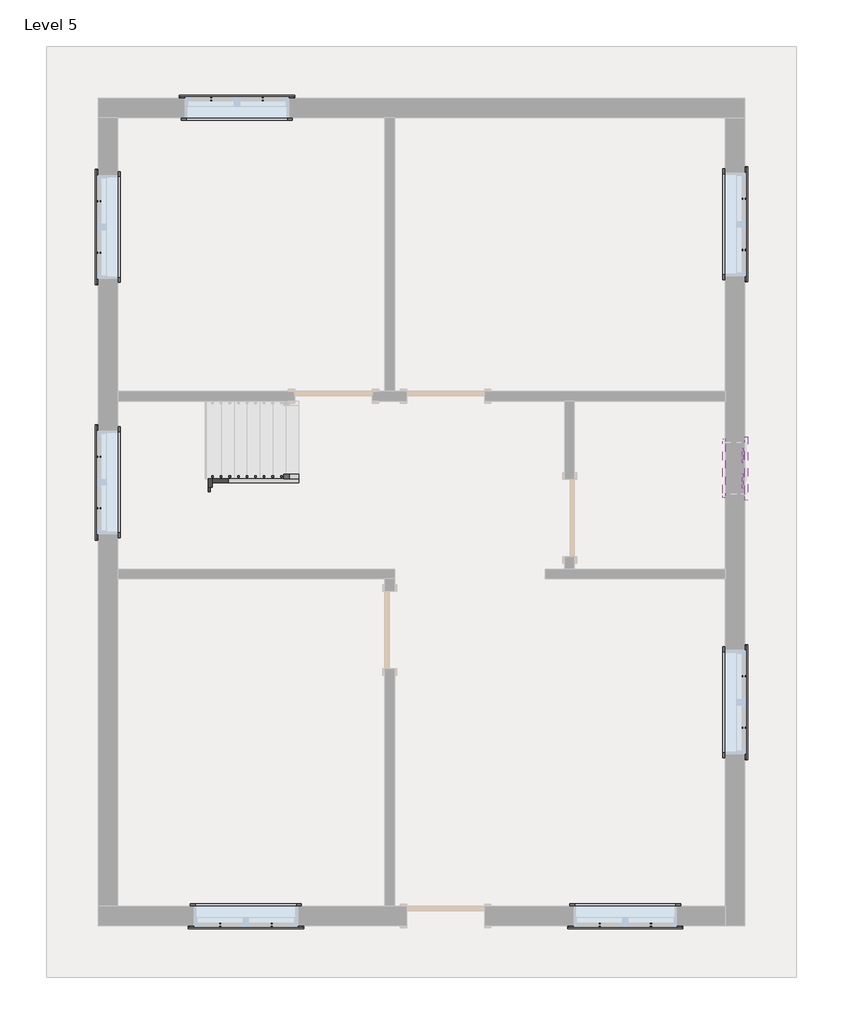
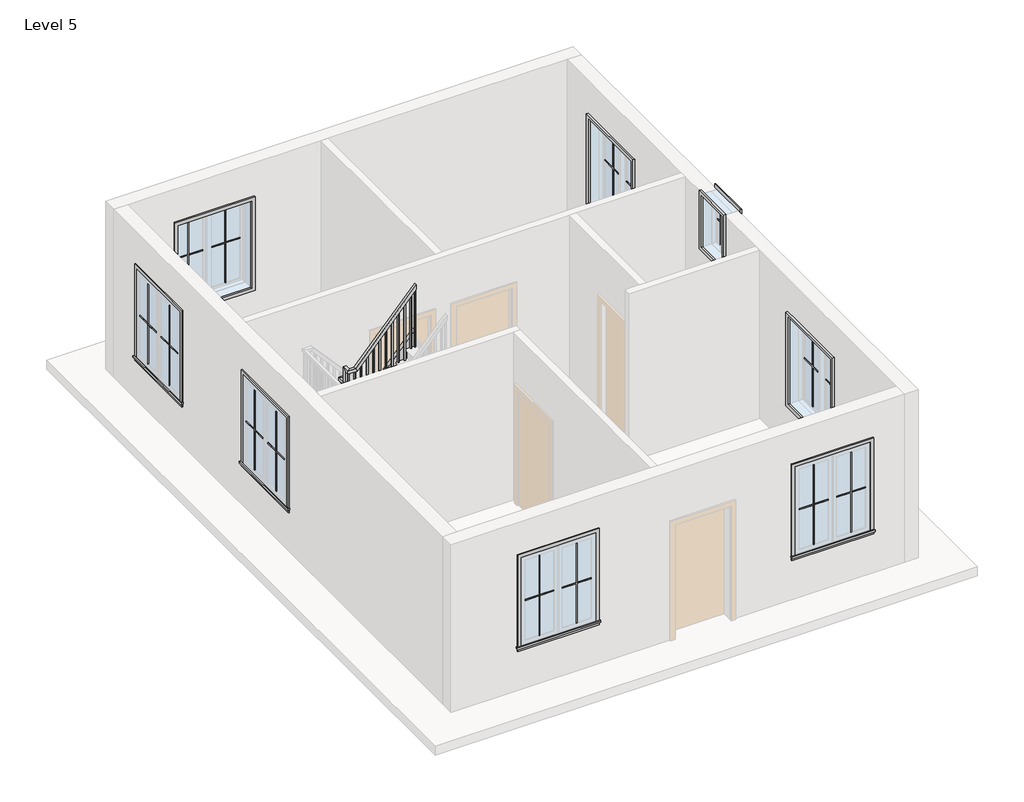
# One storey, part 2 of 2: 32 proxies, 3 members, 1 railing.
"""IFC4 building model written with IfcOpenShell, lengths in millimetres."""

from ifc_helpers import new_model, si_unit, frame, origin, place, context, project, spatial, polyline, outline, extrude, faceted_brep, transform, mapped, element, save
from components import muntin_pattern_2x2_muntin_pattern_2x2_6dad3731, muntin_pattern_2x2_muntin_pattern_2x2_a30a3345, muntin_pattern_2x2_muntin_pattern_2x2_53152e2c, muntin_pattern_2x2_muntin_pattern_2x2_e8f3e573, trim_window_exterior_flat_with_sill_92b9b949, trim_window_exterior_flat_with_sill_a665a915, trim_window_interior_flat_picture_frame_3bb882cf, trim_window_interior_flat_picture_frame_d485c387

model = new_model("IFC4")

# Units and contexts
model_context = context("Model", 3, world=origin())
ifc_project = project(units=[si_unit("LENGTHUNIT", "METRE", prefix="MILLI")], contexts=[model_context])

# Site, building, storey
site = spatial("IfcSite", under=ifc_project)
building = spatial("IfcBuilding", under=site)
storey = spatial("IfcBuildingStorey", under=building, Name="Level 5", Elevation=12192.0)

# Proxies
placement = place(None, origin())
muntin_pattern_2x2_muntin_pattern_2x2_shape = muntin_pattern_2x2_muntin_pattern_2x2_6dad3731(model_context)
element("IfcBuildingElementProxy", 1, Name="Muntin Pattern_2x2 : Muntin Pattern_2x2", ObjectType="Muntin Pattern_2x2 : Muntin Pattern_2x2", at=placement, inside=storey, context=model_context, shape_type="MappedRepresentation", body=[
    mapped(muntin_pattern_2x2_muntin_pattern_2x2_shape, transform((7785.1, 4733.925, 13176.25), x_axis=(-1.0, 0.0, 0.0), y_axis=(0.0, -1.0, 0.0), z_axis=(0.0, 0.0, 1.0))),
])
element("IfcBuildingElementProxy", 2, Name="Muntin Pattern_2x2 : Muntin Pattern_2x2", ObjectType="Muntin Pattern_2x2 : Muntin Pattern_2x2", at=placement, inside=storey, context=model_context, shape_type="MappedRepresentation", body=[
    mapped(muntin_pattern_2x2_muntin_pattern_2x2_shape, transform((3313.1125, 4733.925, 13176.25), x_axis=(-1.0, 0.0, 0.0), y_axis=(0.0, -1.0, 0.0), z_axis=(0.0, 0.0, 1.0))),
])
element("IfcBuildingElementProxy", 3, Name="Muntin Pattern_2x2 : Muntin Pattern_2x2", ObjectType="Muntin Pattern_2x2 : Muntin Pattern_2x2", at=placement, inside=storey, context=model_context, shape_type="MappedRepresentation", body=[
    mapped(muntin_pattern_2x2_muntin_pattern_2x2_shape, transform((8880.475, 13295.3125, 13176.25), x_axis=(0.0, -1.0, 0.0), y_axis=(1.0, 0.0, 0.0), z_axis=(0.0, 0.0, 1.0))),
])
element("IfcBuildingElementProxy", 4, Name="Muntin Pattern_2x2 : Muntin Pattern_2x2", ObjectType="Muntin Pattern_2x2 : Muntin Pattern_2x2", at=placement, inside=storey, context=model_context, shape_type="MappedRepresentation", body=[
    mapped(muntin_pattern_2x2_muntin_pattern_2x2_shape, transform((8880.475, 7662.8625, 13176.25), x_axis=(0.0, -1.0, 0.0), y_axis=(1.0, 0.0, 0.0), z_axis=(0.0, 0.0, 1.0))),
])
element("IfcBuildingElementProxy", 5, Name="Muntin Pattern_2x2 : Muntin Pattern_2x2", ObjectType="Muntin Pattern_2x2 : Muntin Pattern_2x2", at=placement, inside=storey, context=model_context, shape_type="MappedRepresentation", body=[
    mapped(muntin_pattern_2x2_muntin_pattern_2x2_shape, transform((1279.525, 12657.1375, 13176.25), x_axis=(0.0, 1.0, 0.0), y_axis=(-1.0, 0.0, 0.0), z_axis=(0.0, 0.0, 1.0))),
])
element("IfcBuildingElementProxy", 6, Name="Muntin Pattern_2x2 : Muntin Pattern_2x2", ObjectType="Muntin Pattern_2x2 : Muntin Pattern_2x2", at=placement, inside=storey, context=model_context, shape_type="MappedRepresentation", body=[
    mapped(muntin_pattern_2x2_muntin_pattern_2x2_shape, transform((1279.525, 9647.2375, 13176.25), x_axis=(0.0, 1.0, 0.0), y_axis=(-1.0, 0.0, 0.0), z_axis=(0.0, 0.0, 1.0))),
])
element("IfcBuildingElementProxy", 7, Name="Muntin Pattern_2x2 : Muntin Pattern_2x2", ObjectType="Muntin Pattern_2x2 : Muntin Pattern_2x2", at=placement, inside=storey, context=model_context, shape_type="MappedRepresentation", body=[
    mapped(muntin_pattern_2x2_muntin_pattern_2x2_shape, transform((2601.9125, 14468.475, 13176.25), x_axis=(1.0, 0.0, 0.0), y_axis=(0.0, 1.0, 0.0), z_axis=(0.0, 0.0, 1.0))),
])
muntin_pattern_2x2_muntin_pattern_2x2_2_shape = muntin_pattern_2x2_muntin_pattern_2x2_a30a3345(model_context)
element("IfcBuildingElementProxy", 8, Name="Muntin Pattern_2x2 : Muntin Pattern_2x2", ObjectType="Muntin Pattern_2x2 : Muntin Pattern_2x2", at=placement, inside=storey, context=model_context, shape_type="MappedRepresentation", body=[
    mapped(muntin_pattern_2x2_muntin_pattern_2x2_2_shape, transform((7178.675, 4733.925, 13176.25), x_axis=(1.0, 0.0, 0.0), y_axis=(0.0, 1.0, 0.0), z_axis=(0.0, 0.0, 1.0))),
])
element("IfcBuildingElementProxy", 9, Name="Muntin Pattern_2x2 : Muntin Pattern_2x2", ObjectType="Muntin Pattern_2x2 : Muntin Pattern_2x2", at=placement, inside=storey, context=model_context, shape_type="MappedRepresentation", body=[
    mapped(muntin_pattern_2x2_muntin_pattern_2x2_2_shape, transform((2706.6875, 4733.925, 13176.25), x_axis=(1.0, 0.0, 0.0), y_axis=(0.0, 1.0, 0.0), z_axis=(0.0, 0.0, 1.0))),
])
element("IfcBuildingElementProxy", 10, Name="Muntin Pattern_2x2 : Muntin Pattern_2x2", ObjectType="Muntin Pattern_2x2 : Muntin Pattern_2x2", at=placement, inside=storey, context=model_context, shape_type="MappedRepresentation", body=[
    mapped(muntin_pattern_2x2_muntin_pattern_2x2_2_shape, transform((8880.475, 12688.8875, 13176.25), x_axis=(0.0, 1.0, 0.0), y_axis=(-1.0, 0.0, 0.0), z_axis=(0.0, 0.0, 1.0))),
])
element("IfcBuildingElementProxy", 11, Name="Muntin Pattern_2x2 : Muntin Pattern_2x2", ObjectType="Muntin Pattern_2x2 : Muntin Pattern_2x2", at=placement, inside=storey, context=model_context, shape_type="MappedRepresentation", body=[
    mapped(muntin_pattern_2x2_muntin_pattern_2x2_2_shape, transform((8880.475, 7056.4375, 13176.25), x_axis=(0.0, 1.0, 0.0), y_axis=(-1.0, 0.0, 0.0), z_axis=(0.0, 0.0, 1.0))),
])
element("IfcBuildingElementProxy", 12, Name="Muntin Pattern_2x2 : Muntin Pattern_2x2", ObjectType="Muntin Pattern_2x2 : Muntin Pattern_2x2", at=placement, inside=storey, context=model_context, shape_type="MappedRepresentation", body=[
    mapped(muntin_pattern_2x2_muntin_pattern_2x2_2_shape, transform((1279.525, 13263.5625, 13176.25), x_axis=(0.0, -1.0, 0.0), y_axis=(1.0, 0.0, 0.0), z_axis=(0.0, 0.0, 1.0))),
])
element("IfcBuildingElementProxy", 13, Name="Muntin Pattern_2x2 : Muntin Pattern_2x2", ObjectType="Muntin Pattern_2x2 : Muntin Pattern_2x2", at=placement, inside=storey, context=model_context, shape_type="MappedRepresentation", body=[
    mapped(muntin_pattern_2x2_muntin_pattern_2x2_2_shape, transform((1279.525, 10253.6625, 13176.25), x_axis=(0.0, -1.0, 0.0), y_axis=(1.0, 0.0, 0.0), z_axis=(0.0, 0.0, 1.0))),
])
element("IfcBuildingElementProxy", 14, Name="Muntin Pattern_2x2 : Muntin Pattern_2x2", ObjectType="Muntin Pattern_2x2 : Muntin Pattern_2x2", at=placement, inside=storey, context=model_context, shape_type="MappedRepresentation", body=[
    mapped(muntin_pattern_2x2_muntin_pattern_2x2_2_shape, transform((3208.3375, 14468.475, 13176.25), x_axis=(-1.0, 0.0, 0.0), y_axis=(0.0, -1.0, 0.0), z_axis=(0.0, 0.0, 1.0))),
])
muntin_pattern_2x2_muntin_pattern_2x2_3_shape = muntin_pattern_2x2_muntin_pattern_2x2_53152e2c(model_context)
element("IfcBuildingElementProxy", 15, Name="Muntin Pattern_2x2 : Muntin Pattern_2x2", ObjectType="Muntin Pattern_2x2 : Muntin Pattern_2x2", at=placement, inside=storey, context=model_context, shape_type="MappedRepresentation", body=[
    mapped(muntin_pattern_2x2_muntin_pattern_2x2_3_shape, transform((8880.475, 10266.3625, 14395.45), x_axis=(0.0, -1.0, 0.0), y_axis=(1.0, 0.0, 0.0), z_axis=(0.0, 0.0, 1.0))),
])
muntin_pattern_2x2_muntin_pattern_2x2_4_shape = muntin_pattern_2x2_muntin_pattern_2x2_e8f3e573(model_context)
element("IfcBuildingElementProxy", 16, Name="Muntin Pattern_2x2 : Muntin Pattern_2x2", ObjectType="Muntin Pattern_2x2 : Muntin Pattern_2x2", at=placement, inside=storey, context=model_context, shape_type="MappedRepresentation", body=[
    mapped(muntin_pattern_2x2_muntin_pattern_2x2_4_shape, transform((8880.475, 9964.7375, 14395.45), x_axis=(0.0, 1.0, 0.0), y_axis=(-1.0, 0.0, 0.0), z_axis=(0.0, 0.0, 1.0))),
])
trim_window_exterior_flat_with_sill_shape = trim_window_exterior_flat_with_sill_92b9b949(model_context)
element("IfcBuildingElementProxy", 17, Name="Trim-Window-Exterior-Flat : with Sill", ObjectType="Trim-Window-Exterior-Flat : with Sill", at=placement, inside=storey, context=model_context, shape_type="MappedRepresentation", body=[
    mapped(trim_window_exterior_flat_with_sill_shape, transform((7481.8875, 4724.4, 14630.4), x_axis=(1.0, 0.0, 0.0), y_axis=(0.0, 0.0, 1.0), z_axis=(0.0, -1.0, 0.0))),
])
element("IfcBuildingElementProxy", 18, Name="Trim-Window-Exterior-Flat : with Sill", ObjectType="Trim-Window-Exterior-Flat : with Sill", at=placement, inside=storey, context=model_context, shape_type="MappedRepresentation", body=[
    mapped(trim_window_exterior_flat_with_sill_shape, transform((3009.9, 4724.4, 14630.4), x_axis=(1.0, 0.0, 0.0), y_axis=(0.0, 0.0, 1.0), z_axis=(0.0, -1.0, 0.0))),
])
element("IfcBuildingElementProxy", 19, Name="Trim-Window-Exterior-Flat : with Sill", ObjectType="Trim-Window-Exterior-Flat : with Sill", at=placement, inside=storey, context=model_context, shape_type="MappedRepresentation", body=[
    mapped(trim_window_exterior_flat_with_sill_shape, transform((8890.0, 12992.1, 14630.4), x_axis=(0.0, 1.0, 0.0), y_axis=(0.0, 0.0, 1.0), z_axis=(1.0, 0.0, 0.0))),
])
element("IfcBuildingElementProxy", 20, Name="Trim-Window-Exterior-Flat : with Sill", ObjectType="Trim-Window-Exterior-Flat : with Sill", at=placement, inside=storey, context=model_context, shape_type="MappedRepresentation", body=[
    mapped(trim_window_exterior_flat_with_sill_shape, transform((8890.0, 7359.65, 14630.4), x_axis=(0.0, 1.0, 0.0), y_axis=(0.0, 0.0, 1.0), z_axis=(1.0, 0.0, 0.0))),
])
element("IfcBuildingElementProxy", 21, Name="Trim-Window-Exterior-Flat : with Sill", ObjectType="Trim-Window-Exterior-Flat : with Sill", at=placement, inside=storey, context=model_context, shape_type="MappedRepresentation", body=[
    mapped(trim_window_exterior_flat_with_sill_shape, transform((1270.0, 12960.35, 14630.4), x_axis=(0.0, -1.0, 0.0), y_axis=(0.0, 0.0, 1.0), z_axis=(-1.0, 0.0, 0.0))),
])
element("IfcBuildingElementProxy", 22, Name="Trim-Window-Exterior-Flat : with Sill", ObjectType="Trim-Window-Exterior-Flat : with Sill", at=placement, inside=storey, context=model_context, shape_type="MappedRepresentation", body=[
    mapped(trim_window_exterior_flat_with_sill_shape, transform((1270.0, 9950.45, 14630.4), x_axis=(0.0, -1.0, 0.0), y_axis=(0.0, 0.0, 1.0), z_axis=(-1.0, 0.0, 0.0))),
])
element("IfcBuildingElementProxy", 23, Name="Trim-Window-Exterior-Flat : with Sill", ObjectType="Trim-Window-Exterior-Flat : with Sill", at=placement, inside=storey, context=model_context, shape_type="MappedRepresentation", body=[
    mapped(trim_window_exterior_flat_with_sill_shape, transform((2905.125, 14478.0, 14630.4), x_axis=(-1.0, 0.0, 0.0), y_axis=(0.0, 0.0, 1.0), z_axis=(0.0, 1.0, 0.0))),
])
trim_window_exterior_flat_with_sill_2_shape = trim_window_exterior_flat_with_sill_a665a915(model_context)
element("IfcBuildingElementProxy", 24, Name="Trim-Window-Exterior-Flat : with Sill", ObjectType="Trim-Window-Exterior-Flat : with Sill", at=placement, inside=storey, context=model_context, shape_type="MappedRepresentation", body=[
    mapped(trim_window_exterior_flat_with_sill_2_shape, transform((8890.0, 10115.55, 15240.0), x_axis=(0.0, 1.0, 0.0), y_axis=(0.0, 0.0, 1.0), z_axis=(1.0, 0.0, 0.0))),
])
trim_window_interior_flat_picture_frame_shape = trim_window_interior_flat_picture_frame_3bb882cf(model_context)
element("IfcBuildingElementProxy", 25, Name="Trim-Window-Interior-Flat : Picture Frame", ObjectType="Trim-Window-Interior-Flat : Picture Frame", at=placement, inside=storey, context=model_context, shape_type="MappedRepresentation", body=[
    mapped(trim_window_interior_flat_picture_frame_shape, transform((7481.8875, 4953.0, 14630.4), x_axis=(-1.0, 0.0, 0.0), y_axis=(0.0, 0.0, 1.0), z_axis=(0.0, 1.0, 0.0))),
])
element("IfcBuildingElementProxy", 26, Name="Trim-Window-Interior-Flat : Picture Frame", ObjectType="Trim-Window-Interior-Flat : Picture Frame", at=placement, inside=storey, context=model_context, shape_type="MappedRepresentation", body=[
    mapped(trim_window_interior_flat_picture_frame_shape, transform((3009.9, 4953.0, 14630.4), x_axis=(-1.0, 0.0, 0.0), y_axis=(0.0, 0.0, 1.0), z_axis=(0.0, 1.0, 0.0))),
])
element("IfcBuildingElementProxy", 27, Name="Trim-Window-Interior-Flat : Picture Frame", ObjectType="Trim-Window-Interior-Flat : Picture Frame", at=placement, inside=storey, context=model_context, shape_type="MappedRepresentation", body=[
    mapped(trim_window_interior_flat_picture_frame_shape, transform((8661.4, 12992.1, 14630.4), x_axis=(0.0, -1.0, 0.0), y_axis=(0.0, 0.0, 1.0), z_axis=(-1.0, 0.0, 0.0))),
])
element("IfcBuildingElementProxy", 28, Name="Trim-Window-Interior-Flat : Picture Frame", ObjectType="Trim-Window-Interior-Flat : Picture Frame", at=placement, inside=storey, context=model_context, shape_type="MappedRepresentation", body=[
    mapped(trim_window_interior_flat_picture_frame_shape, transform((8661.4, 7359.65, 14630.4), x_axis=(0.0, -1.0, 0.0), y_axis=(0.0, 0.0, 1.0), z_axis=(-1.0, 0.0, 0.0))),
])
element("IfcBuildingElementProxy", 29, Name="Trim-Window-Interior-Flat : Picture Frame", ObjectType="Trim-Window-Interior-Flat : Picture Frame", at=placement, inside=storey, context=model_context, shape_type="MappedRepresentation", body=[
    mapped(trim_window_interior_flat_picture_frame_shape, transform((1498.6, 12960.35, 14630.4), x_axis=(0.0, 1.0, 0.0), y_axis=(0.0, 0.0, 1.0), z_axis=(1.0, 0.0, 0.0))),
])
element("IfcBuildingElementProxy", 30, Name="Trim-Window-Interior-Flat : Picture Frame", ObjectType="Trim-Window-Interior-Flat : Picture Frame", at=placement, inside=storey, context=model_context, shape_type="MappedRepresentation", body=[
    mapped(trim_window_interior_flat_picture_frame_shape, transform((1498.6, 9950.45, 14630.4), x_axis=(0.0, 1.0, 0.0), y_axis=(0.0, 0.0, 1.0), z_axis=(1.0, 0.0, 0.0))),
])
element("IfcBuildingElementProxy", 31, Name="Trim-Window-Interior-Flat : Picture Frame", ObjectType="Trim-Window-Interior-Flat : Picture Frame", at=placement, inside=storey, context=model_context, shape_type="MappedRepresentation", body=[
    mapped(trim_window_interior_flat_picture_frame_shape, transform((2905.125, 14249.4, 14630.4), x_axis=(1.0, 0.0, 0.0), y_axis=(0.0, 0.0, 1.0), z_axis=(0.0, -1.0, 0.0))),
])
trim_window_interior_flat_picture_frame_2_shape = trim_window_interior_flat_picture_frame_d485c387(model_context)
element("IfcBuildingElementProxy", 32, Name="Trim-Window-Interior-Flat : Picture Frame", ObjectType="Trim-Window-Interior-Flat : Picture Frame", at=placement, inside=storey, context=model_context, shape_type="MappedRepresentation", body=[
    mapped(trim_window_interior_flat_picture_frame_2_shape, transform((8661.4, 10115.55, 15240.0), x_axis=(0.0, -1.0, 0.0), y_axis=(0.0, 0.0, 1.0), z_axis=(-1.0, 0.0, 0.0))),
])

# Members
element("IfcMember", 33, ObjectType="Stringer - 2\" Width", at=placement, inside=storey, context=model_context, shape_type="SweptSolid", body=[
    extrude(outline(polyline([(12192.0, 3632.2), (12466.6288314, 3632.2), (13595.5177203, 2616.2), (13139.8883192, 2616.2), (12192.0, 3469.2994873), (12192.0, 3632.2)])), frame((0.0, 9944.1, 0.0), z_axis=(0.0, 1.0, 0.0), x_axis=(0.0, 0.0, 1.0)), (0.0, 0.0, 1.0), 50.8),
])
element("IfcMember", 34, ObjectType="Stringer - 2\" Width", at=placement, inside=storey, context=model_context, shape_type="SweptSolid", body=[
    extrude(outline(polyline([(2565.4, 9994.9), (2616.2, 9994.9), (2616.2, 9893.3), (2565.4, 9893.3), (2565.4, 9994.9)])), frame((0.0, 0.0, 13318.0666667), z_axis=(0.0, 0.0, 1.0), x_axis=(1.0, 0.0, 0.0)), (0.0, 0.0, 1.0), 304.8),
])
element("IfcMember", 35, ObjectType="Stringer - 2\" Width", at=placement, inside=storey, context=model_context, shape_type="SweptSolid", body=[
    extrude(outline(polyline([(13821.2954981, 2565.4), (13365.666097, 2565.4), (14550.9994303, 3632.2), (15006.6288314, 3632.2), (13821.2954981, 2565.4)])), frame((0.0, 9842.5, 0.0), z_axis=(0.0, 1.0, 0.0), x_axis=(0.0, 0.0, 1.0)), (0.0, 0.0, 1.0), 50.8),
])

# Railing
element("IfcRailing", 36, ObjectType="Handrail - Rectangular", at=placement, inside=storey, context=model_context, shape_type="SolidModel", body=[
    faceted_brep([(3632.2, 9994.9, 13275.7333333), (3632.2, 9994.9, 13199.7950998), (3632.2, 10045.7, 13199.7950998), (3632.2, 10045.7, 13275.7333333), (2641.6, 9994.9, 14376.4), (2590.8, 9994.9, 14356.9062109), (2590.8, 10045.7, 14356.9062109), (2641.6, 10045.7, 14376.4), (2641.6, 9994.9, 14461.0666667), (2590.8, 9994.9, 14410.2666667), (2590.8, 10045.7, 14410.2666667), (2641.6, 10045.7, 14461.0666667), (2565.4, 9994.9, 14461.0666667), (2565.4, 9994.9, 14410.2666667), (2514.6, 10045.7, 14410.2666667), (2514.6, 10045.7, 14461.0666667), (2565.4, 9918.7, 14461.0666667), (2565.4, 9867.9, 14410.2666667), (2514.6, 9867.9, 14410.2666667), (2514.6, 9918.7, 14461.0666667), (2565.4, 9918.7, 14715.0666667), (2565.4, 9867.9, 14664.2666667), (2514.6, 9867.9, 14664.2666667), (2514.6, 9918.7, 14715.0666667), (2565.4, 9842.5, 14715.0666667), (2565.4, 9842.5, 14664.2666667), (2514.6, 9791.7, 14664.2666667), (2514.6, 9791.7, 14715.0666667), (2641.6, 9842.5, 14715.0666667), (2664.2244102, 9842.5, 14664.2666667), (2664.2244102, 9791.7, 14664.2666667), (2641.6, 9791.7, 14715.0666667), (3632.2, 9842.5, 15815.7333333), (3632.2, 9791.7, 15815.7333333), (3632.2, 9791.7, 15739.7950998), (3632.2, 9842.5, 15739.7950998)], [[[0, 1, 2, 3]], [[1, 0, 4, 5]], [[2, 1, 5, 6]], [[3, 2, 6, 7]], [[0, 3, 7, 4]], [[5, 4, 8, 9]], [[6, 5, 9, 10]], [[7, 6, 10, 11]], [[4, 7, 11, 8]], [[9, 8, 12, 13]], [[10, 9, 13, 14]], [[11, 10, 14, 15]], [[8, 11, 15, 12]], [[13, 12, 16, 17]], [[14, 13, 17, 18]], [[15, 14, 18, 19]], [[12, 15, 19, 16]], [[17, 16, 20, 21]], [[18, 17, 21, 22]], [[19, 18, 22, 23]], [[16, 19, 23, 20]], [[21, 20, 24, 25]], [[22, 21, 25, 26]], [[23, 22, 26, 27]], [[20, 23, 27, 24]], [[25, 24, 28, 29]], [[26, 25, 29, 30]], [[27, 26, 30, 31]], [[24, 27, 31, 28]], [[32, 33, 34, 35]], [[29, 28, 32, 35]], [[30, 29, 35, 34]], [[31, 30, 34, 33]], [[28, 31, 33, 32]]]),
    extrude(outline(polyline([(15644.5450998, 3546.475), (14732.0, 3546.475), (14732.0, 3565.525), (15665.7117665, 3565.525), (15644.5450998, 3546.475)])), frame((0.0, 9807.575, 0.0), z_axis=(0.0, 1.0, 0.0), x_axis=(0.0, 0.0, 1.0)), (0.0, 0.0, 1.0), 19.05),
    extrude(outline(polyline([(15531.6562109, 3444.875), (14562.6666667, 3444.875), (14562.6666667, 3463.925), (15552.8228776, 3463.925), (15531.6562109, 3444.875)])), frame((0.0, 9807.575, 0.0), z_axis=(0.0, 1.0, 0.0), x_axis=(0.0, 0.0, 1.0)), (0.0, 0.0, 1.0), 19.05),
    extrude(outline(polyline([(15418.767322, 3343.275), (14562.6666667, 3343.275), (14562.6666667, 3362.325), (15439.9339887, 3362.325), (15418.767322, 3343.275)])), frame((0.0, 9807.575, 0.0), z_axis=(0.0, 1.0, 0.0), x_axis=(0.0, 0.0, 1.0)), (0.0, 0.0, 1.0), 19.05),
    extrude(outline(polyline([(15305.8784332, 3241.675), (14393.3333333, 3241.675), (14393.3333333, 3260.725), (15327.0450998, 3260.725), (15305.8784332, 3241.675)])), frame((0.0, 9807.575, 0.0), z_axis=(0.0, 1.0, 0.0), x_axis=(0.0, 0.0, 1.0)), (0.0, 0.0, 1.0), 19.05),
    extrude(outline(polyline([(15192.9895443, 3140.075), (14224.0, 3140.075), (14224.0, 3159.125), (15214.1562109, 3159.125), (15192.9895443, 3140.075)])), frame((0.0, 9807.575, 0.0), z_axis=(0.0, 1.0, 0.0), x_axis=(0.0, 0.0, 1.0)), (0.0, 0.0, 1.0), 19.05),
    extrude(outline(polyline([(15080.1006554, 3038.475), (14224.0, 3038.475), (14224.0, 3057.525), (15101.267322, 3057.525), (15080.1006554, 3038.475)])), frame((0.0, 9807.575, 0.0), z_axis=(0.0, 1.0, 0.0), x_axis=(0.0, 0.0, 1.0)), (0.0, 0.0, 1.0), 19.05),
    extrude(outline(polyline([(14967.2117665, 2936.875), (14054.6666667, 2936.875), (14054.6666667, 2955.925), (14988.3784332, 2955.925), (14967.2117665, 2936.875)])), frame((0.0, 9807.575, 0.0), z_axis=(0.0, 1.0, 0.0), x_axis=(0.0, 0.0, 1.0)), (0.0, 0.0, 1.0), 19.05),
    extrude(outline(polyline([(14854.3228776, 2835.275), (13885.3333333, 2835.275), (13885.3333333, 2854.325), (14875.4895443, 2854.325), (14854.3228776, 2835.275)])), frame((0.0, 9807.575, 0.0), z_axis=(0.0, 1.0, 0.0), x_axis=(0.0, 0.0, 1.0)), (0.0, 0.0, 1.0), 19.05),
    extrude(outline(polyline([(14741.4339887, 2733.675), (13885.3333333, 2733.675), (13885.3333333, 2752.725), (14762.6006554, 2752.725), (14741.4339887, 2733.675)])), frame((0.0, 9807.575, 0.0), z_axis=(0.0, 1.0, 0.0), x_axis=(0.0, 0.0, 1.0)), (0.0, 0.0, 1.0), 19.05),
    extrude(outline(polyline([(14628.5450998, 2632.075), (13716.0, 2632.075), (13716.0, 2651.125), (14649.7117665, 2651.125), (14628.5450998, 2632.075)])), frame((0.0, 9807.575, 0.0), z_axis=(0.0, 1.0, 0.0), x_axis=(0.0, 0.0, 1.0)), (0.0, 0.0, 1.0), 19.05),
    extrude(outline(polyline([(2549.525, 9928.225), (2549.525, 9909.175), (2530.475, 9909.175), (2530.475, 9928.225), (2549.525, 9928.225)])), frame((0.0, 0.0, 13546.6666667), z_axis=(0.0, 0.0, 1.0), x_axis=(1.0, 0.0, 0.0)), (0.0, 0.0, 1.0), 863.6),
    extrude(outline(polyline([(2625.725, 10010.775), (2606.675, 10010.775), (2606.675, 10029.825), (2625.725, 10029.825), (2625.725, 10010.775)])), frame((0.0, 0.0, 13377.3333333), z_axis=(0.0, 0.0, 1.0), x_axis=(1.0, 0.0, 0.0)), (0.0, 0.0, 1.0), 1032.9333333),
    extrude(outline(polyline([(14226.3784332, 2708.275), (13377.3333333, 2708.275), (13377.3333333, 2727.325), (14205.2117665, 2727.325), (14226.3784332, 2708.275)])), frame((0.0, 10010.775, 0.0), z_axis=(0.0, 1.0, 0.0), x_axis=(0.0, 0.0, 1.0)), (0.0, 0.0, 1.0), 19.05),
    extrude(outline(polyline([(14113.4895443, 2809.875), (13208.0, 2809.875), (13208.0, 2828.925), (14092.3228776, 2828.925), (14113.4895443, 2809.875)])), frame((0.0, 10010.775, 0.0), z_axis=(0.0, 1.0, 0.0), x_axis=(0.0, 0.0, 1.0)), (0.0, 0.0, 1.0), 19.05),
    extrude(outline(polyline([(14000.6006554, 2911.475), (13038.6666667, 2911.475), (13038.6666667, 2930.525), (13979.4339887, 2930.525), (14000.6006554, 2911.475)])), frame((0.0, 10010.775, 0.0), z_axis=(0.0, 1.0, 0.0), x_axis=(0.0, 0.0, 1.0)), (0.0, 0.0, 1.0), 19.05),
    extrude(outline(polyline([(13887.7117665, 3013.075), (13038.6666667, 3013.075), (13038.6666667, 3032.125), (13866.5450998, 3032.125), (13887.7117665, 3013.075)])), frame((0.0, 10010.775, 0.0), z_axis=(0.0, 1.0, 0.0), x_axis=(0.0, 0.0, 1.0)), (0.0, 0.0, 1.0), 19.05),
    extrude(outline(polyline([(13774.8228776, 3114.675), (12869.3333333, 3114.675), (12869.3333333, 3133.725), (13753.6562109, 3133.725), (13774.8228776, 3114.675)])), frame((0.0, 10010.775, 0.0), z_axis=(0.0, 1.0, 0.0), x_axis=(0.0, 0.0, 1.0)), (0.0, 0.0, 1.0), 19.05),
    extrude(outline(polyline([(13661.9339887, 3216.275), (12700.0, 3216.275), (12700.0, 3235.325), (13640.767322, 3235.325), (13661.9339887, 3216.275)])), frame((0.0, 10010.775, 0.0), z_axis=(0.0, 1.0, 0.0), x_axis=(0.0, 0.0, 1.0)), (0.0, 0.0, 1.0), 19.05),
    extrude(outline(polyline([(13549.0450998, 3317.875), (12700.0, 3317.875), (12700.0, 3336.925), (13527.8784332, 3336.925), (13549.0450998, 3317.875)])), frame((0.0, 10010.775, 0.0), z_axis=(0.0, 1.0, 0.0), x_axis=(0.0, 0.0, 1.0)), (0.0, 0.0, 1.0), 19.05),
    extrude(outline(polyline([(13436.1562109, 3419.475), (12530.6666667, 3419.475), (12530.6666667, 3438.525), (13414.9895443, 3438.525), (13436.1562109, 3419.475)])), frame((0.0, 10010.775, 0.0), z_axis=(0.0, 1.0, 0.0), x_axis=(0.0, 0.0, 1.0)), (0.0, 0.0, 1.0), 19.05),
    extrude(outline(polyline([(13323.267322, 3521.075), (12361.3333333, 3521.075), (12361.3333333, 3540.125), (13302.1006554, 3540.125), (13323.267322, 3521.075)])), frame((0.0, 10010.775, 0.0), z_axis=(0.0, 1.0, 0.0), x_axis=(0.0, 0.0, 1.0)), (0.0, 0.0, 1.0), 19.05),
    extrude(outline(polyline([(2549.525, 9826.625), (2549.525, 9807.575), (2530.475, 9807.575), (2530.475, 9826.625), (2549.525, 9826.625)])), frame((0.0, 0.0, 13546.6666667), z_axis=(0.0, 0.0, 1.0), x_axis=(1.0, 0.0, 0.0)), (0.0, 0.0, 1.0), 1117.6),
    extrude(outline(polyline([(2549.525, 10010.775), (2530.475, 10010.775), (2530.475, 10029.825), (2549.525, 10029.825), (2549.525, 10010.775)])), frame((0.0, 0.0, 13546.6666667), z_axis=(0.0, 0.0, 1.0), x_axis=(1.0, 0.0, 0.0)), (0.0, 0.0, 1.0), 863.6),
    extrude(outline(polyline([(15718.6284332, 3613.15), (14732.0, 3613.15), (14732.0, 3632.2), (15739.7950998, 3632.2), (15718.6284332, 3613.15)])), frame((0.0, 9807.575, 0.0), z_axis=(0.0, 1.0, 0.0), x_axis=(0.0, 0.0, 1.0)), (0.0, 0.0, 1.0), 19.05),
    extrude(outline(polyline([(13220.9617665, 3613.15), (12361.3333333, 3613.15), (12361.3333333, 3632.2), (13199.7950998, 3632.2), (13220.9617665, 3613.15)])), frame((0.0, 10010.775, 0.0), z_axis=(0.0, 1.0, 0.0), x_axis=(0.0, 0.0, 1.0)), (0.0, 0.0, 1.0), 19.05),
])

save(model, "model.ifc")

# Revit data of these elements
# Type "Muntin Pattern_2x2 : Muntin Pattern_2x2"
#   Width [instance default] = 4' - 0"
#   Thickness = 0' - 0 1/2"
#   Height [instance default] = 4' - 0"
#   Distance = 0' - 0 3/4"
#   Interior Material [instance default] = none
#   Exterior Material [instance default] = none
#   Default Elevation = 0
# Type "Trim-Window-Exterior-Flat : with Sill"
#   Trim Width = 0' - 2 1/4"
#   Trim Thickness_Picture Frame = 0' - 1 1/4"
#   Trim Thickness_with Sill = 0' - 0 3/4"
#   Sill Thickness = 0' - 1 1/4"
#   Opening Width [instance default] = 2' - 0"
#   Opening Height [instance default] = 3' - 0"
#   Default Elevation = 4' - 0"
#   Sill = yes
#   Picture Frame = no
#   Trim Material [instance default] = none
# Type "Trim-Window-Interior-Flat : Picture Frame"
#   Trim Thickness_Picture Frame = 0' - 1 1/4"
#   Trim Width = 0' - 2 1/4"
#   Trim Thickness_with Sill = 0' - 0 3/4"
#   Sill Thickness = 0' - 1 1/4"
#   Opening Width [instance default] = 2' - 0"
#   Opening Height [instance default] = 3' - 0"
#   Default Elevation = 4' - 0"
#   Sill = no
#   Picture Frame = yes
#   Trim Material [instance default] = none
# Type "Handrail - Rectangular"
#   Assembly Code = "C2010400"
#   built-in parameter 1008612 = 0.0416667 (stored number, unit not read)
#   built-in parameter 1008611 = 0.0416667 (stored number, unit not read)
#   built-in parameter 1008609 = 0.333333 (stored number, unit not read)
#   built-in parameter 1008604 = 0.166667 (stored number, unit not read)
#   built-in parameter 1008603 = 0.166667 (stored number, unit not read)
#   Railing Height = 3' - 0"
#   built-in parameter 1008630 = 2
#   built-in parameter 1008610 = 2
#   built-in parameter 1008618 = Baluster - Square : 3/4"
# Elements 1, 2, 3, 4, 5, 6, 7, 8, 9, 10, 11, 12, 13, 14 (IfcBuildingElementProxy, "Muntin Pattern_2x2 : Muntin Pattern_2x2")
#   Width = 1' - 6 5/8"
#   Height = 4' - 6 1/2"
#   Interior Material = Wood - Stained
#   Exterior Material = Clad - White
#   Phase Created = New Construction
#   Materials on its faces: "Clad - White", "Wood - Stained"
# Elements 15, 16 (IfcBuildingElementProxy, "Muntin Pattern_2x2 : Muntin Pattern_2x2")
#   Width = 0' - 6 5/8"
#   Height = 2' - 6 1/2"
#   Interior Material = Wood - Stained
#   Exterior Material = Clad - White
#   Phase Created = New Construction
#   Materials on its faces: "Clad - White", "Wood - Stained"
# Elements 17, 18, 19, 20, 21, 22, 23 (IfcBuildingElementProxy, "Trim-Window-Exterior-Flat : with Sill")
#   Opening Width = 4' - 0"
#   Opening Height = 5' - 0"
#   Trim Material = Clad - White
#   Phase Created = New Construction
#   Materials on its faces: "Clad - White"
# Element 24 (IfcBuildingElementProxy, "Trim-Window-Exterior-Flat : with Sill")
#   Opening Width = 2' - 0"
#   Opening Height = 3' - 0"
#   Trim Material = Clad - White
#   Phase Created = New Construction
#   Materials on its faces: "Clad - White"
# Elements 25, 26, 27, 28, 29, 30, 31 (IfcBuildingElementProxy, "Trim-Window-Interior-Flat : Picture Frame")
#   Opening Width = 4' - 0"
#   Opening Height = 5' - 0"
#   Trim Material = Wood - Stained
#   Phase Created = New Construction
#   Materials on its faces: "Wood - Stained"
# Element 32 (IfcBuildingElementProxy, "Trim-Window-Interior-Flat : Picture Frame")
#   Opening Width = 2' - 0"
#   Opening Height = 3' - 0"
#   Trim Material = Wood - Stained
#   Phase Created = New Construction
#   Materials on its faces: "Wood - Stained"
# Elements 33, 34, 35 (IfcMember, "Stringer - 2\" Width")
#   Phase Created = New Construction
# Element 36 (IfcRailing, "Handrail - Rectangular")
#   Phase Created = New Construction
# Materials
#   "Clad - White": class "Wood", colour RGB 242 242 238, transparency 0, Cost = 0
#   "Wood - Stained": class "Wood", colour RGB 224 178 126, transparency 0, Cost = 0
